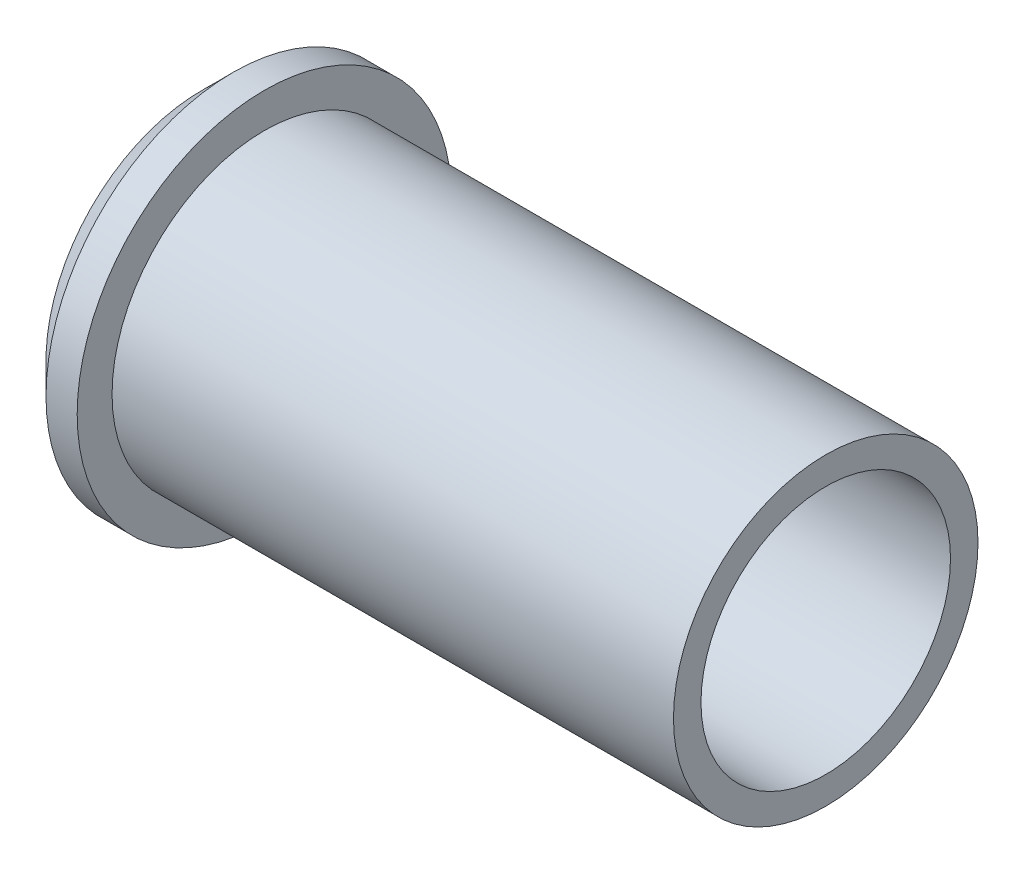
SolidWorks part; units mm, degrees
material "Plain Carbon Steel"
ref_plane "Front Plane" through (0, 0, 0) normal (0, 0, 1) x (1, 0, 0)
ref_plane "Top Plane" through (0, 0, 0) normal (0, 1, 0) x (1, 0, 0)
ref_plane "Right Plane" through (0, 0, 0) normal (1, 0, 0) x (0, 0, -1)
sketch "Bushing Profile Sketch" plane through (0, 0, 0) normal (0, 0, 1) x (1, 0, 0)
  line L0 (40.7811, 0) -> (-45.673, 0) construction
  line L1 (15.875, 6.35) -> (-15.875, 6.35)
  line L2 (-15.875, 6.35) -> (-15.875, 8.89)
  line L4 (-14.2875, 9.525) -> (-12.7, 9.525)
  line L5 (-12.7, 9.525) -> (-12.7, 7.75)
  line L6 (-12.7, 7.75) -> (15.875, 7.75)
  line L7 (15.875, 7.75) -> (15.875, 6.35)
  line L8 (-15.875, 8.89) -> (-15.875, 9.525)
  line L9 (-15.875, 9.525) -> (-14.2875, 9.525)
  dimension "D1" = 6.35
  dimension "D2" = 7.75
  dimension "D3" = 3.175
  dimension "D4" = 1.5875
  dimension "D5" = 9.525
  dimension "D6" = 8.89
  dimension "D7" = 15.875
  dimension "D8" = 31.75
revolve "Flanged Bushing Revolve" add sketch "Bushing Profile Sketch" angle 360 about L0
chamfer "Edge Chamfer 0.0625in x 45deg" distance 1.5875 angle 45 1 edges at (-15.875, 0, -9.525)
